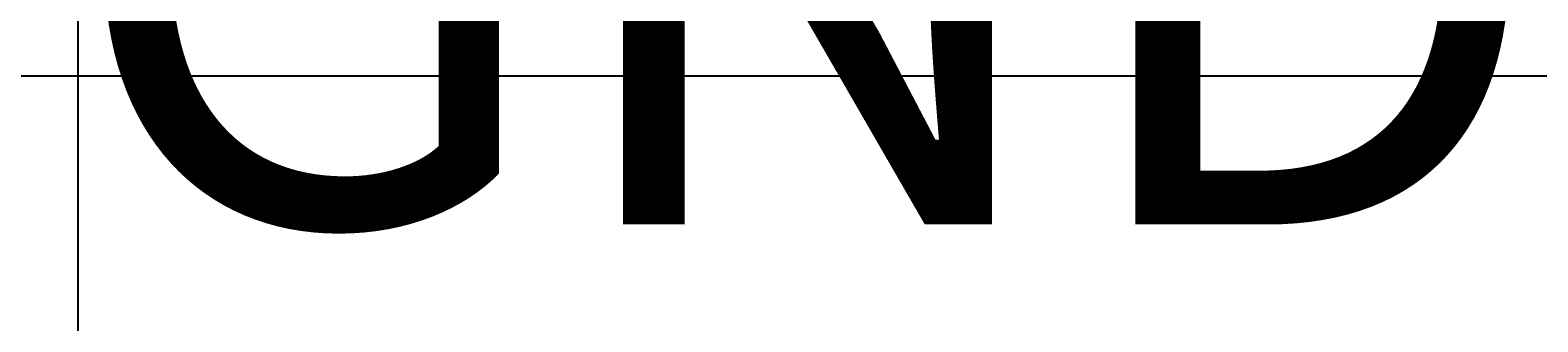
# Model space of a CAD drawing. Units: inches. Extents: x 35362 to 73946, y 43607 to 67532.
# Tile 95 of 134: x 50119 to 50761, y 48793 to 48917. Entities that reach past the tile are written whole.
import ezdxf

# ---------------------------------------------------------------- set-up
doc = ezdxf.new("R2010")
doc.units = ezdxf.units.IN
doc.header["$MEASUREMENT"] = 0
doc.layers.add('A-ANNO-DIMS', color=2, linetype='Continuous', lineweight=18)
doc.layers.add('E-ANNO-TEXT', color=5, linetype='Continuous', lineweight=18)
doc.styles.get("Standard").update_dxf_attribs({"font": 'arial.ttf'})
doc.dimstyles.get("Standard").update_dxf_attribs({"dimtxt": 0.18, "dimasz": 0.18, "dimexe": 0.18, "dimexo": 0.0625, "dimgap": 0.09, "dimtad": 0, "dimtih": 1, "dimtoh": 1, "dimdec": 4, "dimzin": 0, "dimdsep": 46, "dimtxsty": 'Standard', "dimcen": 0.09, "dimadec": 0, "dimazin": 0, "dimtfac": 1, "dimtdec": 4, "dimtofl": 0, "dimtmove": 0, "dimatfit": 3, "dimfxl": 1, "dimtolj": 1, "dimtzin": 0, "dimarcsym": 0})

# ---------------------------------------------------------------- blocks, each defined once
blk = doc.blocks.new('*D11')
at = {"layer": 'A-ANNO-DIMS', "color": 0, "lineweight": -2, "transparency": 16777216}
for p, q in [((47978.66, 56028.77), (47978.66, 43606.68)), ((53109.76, 56028.77), (53109.76, 43606.68)), ((47978.84, 43606.86), (50543.87, 43606.86)), ((53109.58, 43606.86), (50544.55, 43606.86))]:
    blk.add_line(p, q, dxfattribs=at)
at = {"layer": 'A-ANNO-DIMS', "color": 0, "transparency": 16777216}
for points in [[(47978.84, 43606.89), (47978.84, 43606.83), (47978.66, 43606.86)], [(53109.58, 43606.89), (53109.58, 43606.83), (53109.76, 43606.86)]]:
    blk.add_solid(points, dxfattribs=at)
at = {"layer": 'Defpoints', "color": 0, "transparency": 16777216}
for p in [(47978.66, 56028.84), (53109.76, 56028.84), (53109.76, 43606.86)]:
    blk.add_point(p, dxfattribs=at)
at = {"layer": 'A-ANNO-DIMS', "color": 0, "transparency": 16777216, "insert": (50544.21, 43606.86), "char_height": 0.18, "attachment_point": 5}
blk.add_mtext('\\A1;5131', dxfattribs=at)
blk = doc.blocks.new('*D13')
at = {"layer": 'A-ANNO-DIMS', "color": 0, "lineweight": -2, "transparency": 16777216}
for p, q in [((48373.49, 51694.02), (48373.49, 43606.68)), ((51029.04, 51694.02), (51029.04, 43606.68)), ((48373.67, 43606.86), (49700.8, 43606.86)), ((51028.86, 43606.86), (49701.73, 43606.86))]:
    blk.add_line(p, q, dxfattribs=at)
at = {"layer": 'A-ANNO-DIMS', "color": 0, "transparency": 16777216}
for points in [[(48373.67, 43606.89), (48373.67, 43606.83), (48373.49, 43606.86)], [(51028.86, 43606.89), (51028.86, 43606.83), (51029.04, 43606.86)]]:
    blk.add_solid(points, dxfattribs=at)
at = {"layer": 'Defpoints', "color": 0, "transparency": 16777216}
for p in [(48373.49, 51694.09), (51029.04, 51694.09), (51029.04, 43606.86)]:
    blk.add_point(p, dxfattribs=at)
at = {"layer": 'A-ANNO-DIMS', "color": 0, "transparency": 16777216, "insert": (49701.27, 43606.86), "char_height": 0.18, "attachment_point": 5}
blk.add_mtext('\\A1;2655.6', dxfattribs=at)
blk = doc.blocks.new('*D17')
at = {"layer": 'A-ANNO-DIMS', "color": 0, "lineweight": -2, "transparency": 16777216}
for p, q in [((49923.31, 61293.22), (49923.31, 43606.68)), ((51913.93, 61293.22), (51913.93, 43606.68)), ((49923.49, 43606.86), (50918.16, 43606.86)), ((51913.75, 43606.86), (50919.07, 43606.86))]:
    blk.add_line(p, q, dxfattribs=at)
at = {"layer": 'A-ANNO-DIMS', "color": 0, "transparency": 16777216}
for points in [[(49923.49, 43606.89), (49923.49, 43606.83), (49923.31, 43606.86)], [(51913.75, 43606.89), (51913.75, 43606.83), (51913.93, 43606.86)]]:
    blk.add_solid(points, dxfattribs=at)
at = {"layer": 'Defpoints', "color": 0, "transparency": 16777216}
for p in [(49923.31, 61293.29), (51913.93, 61293.29), (51913.93, 43606.86)]:
    blk.add_point(p, dxfattribs=at)
at = {"layer": 'A-ANNO-DIMS', "color": 0, "transparency": 16777216, "insert": (50918.62, 43606.86), "char_height": 0.18, "attachment_point": 5}
blk.add_mtext('\\A1;1990.6', dxfattribs=at)
blk = doc.blocks.new('*D67')
at = {"layer": 'A-ANNO-DIMS', "color": 0, "lineweight": -2, "transparency": 16777216}
for p, q in [((56873.54, 53351.53), (35361.77, 53351.53)), ((35361.95, 53351.35), (35361.95, 49400.89)), ((35361.95, 45450.07), (35361.95, 49400.53)), ((53793.58, 45449.89), (35361.77, 45449.89))]:
    blk.add_line(p, q, dxfattribs=at)
at = {"layer": 'A-ANNO-DIMS', "color": 0, "transparency": 16777216}
for points in [[(35361.92, 53351.35), (35361.98, 53351.35), (35361.95, 53351.53)], [(35361.92, 45450.07), (35361.98, 45450.07), (35361.95, 45449.89)]]:
    blk.add_solid(points, dxfattribs=at)
at = {"layer": 'Defpoints', "color": 0, "transparency": 16777216}
for p in [(35361.95, 53351.53), (56873.6, 53351.53), (53793.64, 45449.89)]:
    blk.add_point(p, dxfattribs=at)
at = {"layer": 'A-ANNO-DIMS', "color": 0, "transparency": 16777216, "insert": (35361.95, 49400.71), "char_height": 0.18, "attachment_point": 5}
blk.add_mtext('\\A1;7901.6', dxfattribs=at)
blk = doc.blocks.new('*D89')
at = {"layer": 'A-ANNO-DIMS', "color": 0, "lineweight": -2, "transparency": 16777216}
for p, q in [((53707.72, 48897.74), (35361.77, 48897.74)), ((35361.95, 48897.56), (35361.95, 48303.16)), ((35361.95, 47708.4), (35361.95, 48302.8)), ((53707.72, 47708.22), (35361.77, 47708.22))]:
    blk.add_line(p, q, dxfattribs=at)
at = {"layer": 'A-ANNO-DIMS', "color": 0, "transparency": 16777216}
for points in [[(35361.92, 48897.56), (35361.98, 48897.56), (35361.95, 48897.74)], [(35361.92, 47708.4), (35361.98, 47708.4), (35361.95, 47708.22)]]:
    blk.add_solid(points, dxfattribs=at)
at = {"layer": 'Defpoints', "color": 0, "transparency": 16777216}
for p in [(53707.78, 48897.74), (35361.95, 47708.22), (53707.78, 47708.22)]:
    blk.add_point(p, dxfattribs=at)
at = {"layer": 'A-ANNO-DIMS', "color": 0, "transparency": 16777216, "insert": (35361.95, 48302.98), "char_height": 0.18, "attachment_point": 5}
blk.add_mtext('\\A1;1189.5', dxfattribs=at)
blk = doc.blocks.new('*D107')
at = {"layer": 'A-ANNO-DIMS', "color": 0, "lineweight": -2, "transparency": 16777216}
for p, q in [((50139.56, 59850.01), (50139.56, 43606.68)), ((51320.81, 59850.01), (51320.81, 43606.68)), ((50139.74, 43606.86), (50729.73, 43606.86)), ((51320.63, 43606.86), (50730.64, 43606.86))]:
    blk.add_line(p, q, dxfattribs=at)
at = {"layer": 'A-ANNO-DIMS', "color": 0, "transparency": 16777216}
for points in [[(50139.74, 43606.89), (50139.74, 43606.83), (50139.56, 43606.86)], [(51320.63, 43606.89), (51320.63, 43606.83), (51320.81, 43606.86)]]:
    blk.add_solid(points, dxfattribs=at)
at = {"layer": 'Defpoints', "color": 0, "transparency": 16777216}
for p in [(50139.56, 59850.08), (51320.81, 59850.08), (51320.81, 43606.86)]:
    blk.add_point(p, dxfattribs=at)
at = {"layer": 'A-ANNO-DIMS', "color": 0, "transparency": 16777216, "insert": (50730.19, 43606.86), "char_height": 0.18, "attachment_point": 5}
blk.add_mtext('\\A1;1181.3', dxfattribs=at)

msp = doc.modelspace()

# ---------------------------------------------------------------- texts
at = {"layer": 'E-ANNO-TEXT'}
msp.add_text('GND', height=220.866, dxfattribs=at).set_placement((50133.331, 48834.598))

# ---------------------------------------------------------------- dimensions: what is measured, and where the dimension line sits
at = {"layer": 'A-ANNO-DIMS'}
for base, p1, p2, override, picture, middle in [((51913.931, 43606.859), (49923.307, 61293.286), (51913.931, 61293.286), {"dimdec": 1, "dimlfac": 1, "dimrnd": 0, "dimzin": 0, "dimdsep": 46, "dimlunit": 2}, '*D17', (50918.619, 43606.859)), ((51320.8133, 43606.859), (50139.5627, 59850.0769), (51320.8133, 59850.0769), {"dimdec": 1, "dimlfac": 1, "dimrnd": 0, "dimzin": 0, "dimdsep": 46, "dimlunit": 2}, '*D107', (50730.188, 43606.859)), ((53109.76, 43606.859), (47978.665, 56028.836), (53109.76, 56028.836), {"dimdec": 0, "dimlfac": 1, "dimrnd": 0, "dimzin": 0, "dimdsep": 46, "dimlunit": 2}, '*D11', (50544.212, 43606.859)), ((51029.043, 43606.859), (48373.492, 51694.087), (51029.043, 51694.087), {"dimdec": 1, "dimlfac": 1, "dimrnd": 0, "dimzin": 0, "dimdsep": 46, "dimlunit": 2}, '*D13', (49701.267, 43606.859))]:
    dim = msp.add_linear_dim(base=base, p1=p1, p2=p2, dimstyle='Standard', override=override, dxfattribs=at)
    dim.commit()
    dim.dimension.update_dxf_attribs({"geometry": picture, "text_midpoint": middle})
for base, p1, p2, picture, middle in [((35361.949, 53351.529), (53793.638, 45449.894), (56873.602, 53351.529), '*D67', (35361.949, 49400.712)), ((35361.949, 47708.216), (53707.781, 48897.738), (53707.781, 47708.216), '*D89', (35361.949, 48302.977))]:
    dim = msp.add_linear_dim(base=base, p1=p1, p2=p2, angle=90, dimstyle='Standard', override={"dimdec": 1, "dimlfac": 1, "dimrnd": 0, "dimzin": 0, "dimdsep": 46, "dimlunit": 2}, dxfattribs=at)
    dim.commit()
    dim.dimension.update_dxf_attribs({"geometry": picture, "text_midpoint": middle})

doc.saveas('drawing.dxf')
